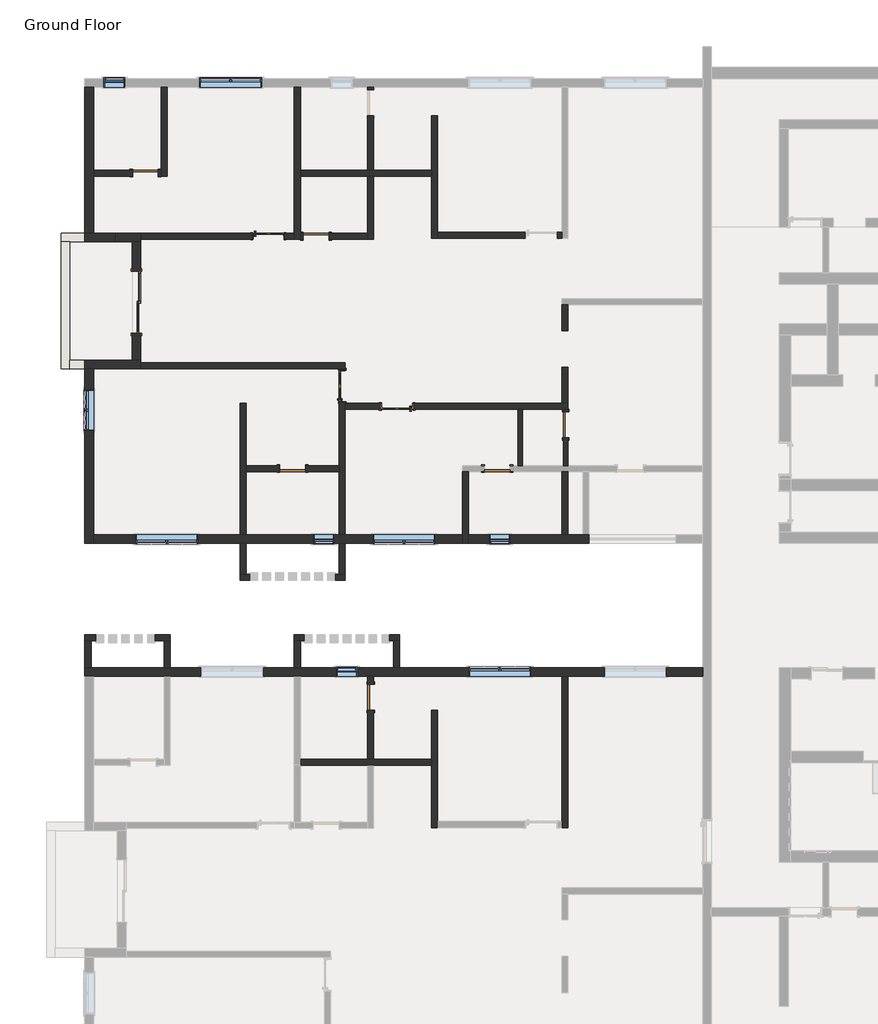
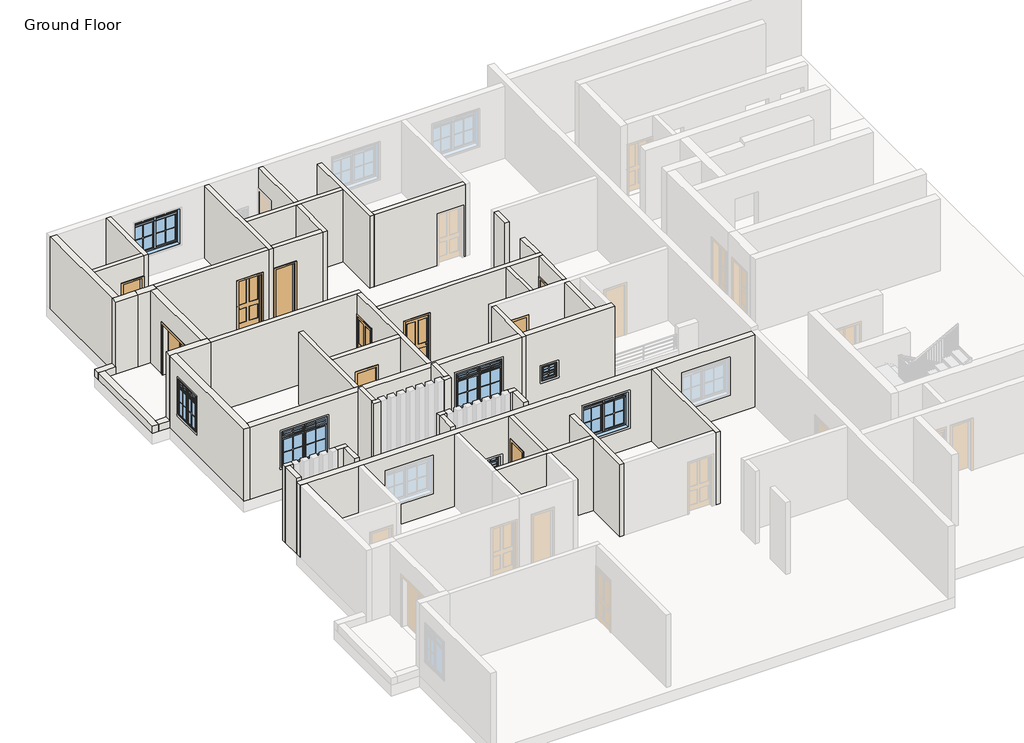
# One storey, part 2 of 9: 49 walls, 10 doors, 9 windows.
# Revit data of these elements (continued)
# Elements 13, 14, 19, 25, 28, 29, 31, 34, 38, 39, 42, 43, 46, 47 (IfcWall, "6\" INTERIOR WALL")
#   Top Offset = 0' - 0"
#   Base Offset = 0' - 0"
#   wall height = 10' - 6"
#   Phase Created = New Construction
#   Base Constraint = Ground Floor
#   Top Constraint = 1st Floor
#   Materials on its faces: "0 Cream", "Default Wall"
# Elements 15, 16, 17, 18, 20, 21, 22, 23, 24, 26, 27, 30, 32, 33, 35, 36, 37, 40, 41, 44, 45 (IfcWall, "6\" INTERIOR WALL")
#   Top Offset = 0' - 0"
#   Base Offset = 0' - 0"
#   wall height = 10' - 6"
#   Phase Created = New Construction
#   Base Constraint = Ground Floor
#   Top Constraint = 1st Floor
#   Materials on its faces: "Default Wall", "0 Cream"
# Elements 48, 49, 50, 51, 54, 55, 59 (IfcWall, "9\" EXTERIOR WALL")
#   Top Offset = 0' - 0"
#   Base Offset = 0' - 0"
#   wall height = 10' - 6"
#   Phase Created = New Construction
#   Base Constraint = Ground Floor
#   Top Constraint = 1st Floor
#   Materials on its faces: "Default Wall", "0 Cream"
# Element 52 (IfcWall, "9\" EXTERIOR WALL")
#   Top Offset = 0' - 0"
#   Base Offset = 0' - 0"
#   Unconnected Height = 1' - 0"
#   wall height = 1' - 0"
#   Phase Created = New Construction
#   Base Constraint = Ground Floor
#   Materials on its faces: "Default Wall", "0 Cream"
# Elements 53, 58 (IfcWall, "9\" EXTERIOR WALL")
#   Top Offset = 0' - 0"
#   Base Offset = 0' - 0"
#   wall height = 10' - 6"
#   Phase Created = New Construction
#   Base Constraint = Ground Floor
#   Top Constraint = 1st Floor
#   Materials on its faces: "0 Cream", "Default Wall"
# Elements 56, 57 (IfcWall, "9\" EXTERIOR WALL")
#   Top Offset = 0' - 0"
#   Base Offset = 0' - 0"
#   Unconnected Height = 1' - 0"
#   wall height = 1' - 0"
#   Phase Created = New Construction
#   Base Constraint = Ground Floor
#   Materials on its faces: "0 Cream", "Default Wall"
# Element 60 (IfcWindow, "Window-Casement-Double-Awning-Double : 4' x 5' Window")
#   Mark = "29"
#   Window Inset = 0' - 0"
#   Interior Wall Closure = 0' - 2 1/4"
#   Frame Extension = 0' - 0 1/4"
#   Exterior Wall Closure = 0' - 1 1/4"
#   Interior Trim Visibility = yes
#   Exterior Trim Visibility = yes
#   Phase Created = New Construction
#   Materials on its faces: "Wood - Stained", "Glass", "Clad - White"
# Element 61 (IfcWindow, "Window-Casement-Double-Awning-Double : 6' x 5'")
#   Mark = "5"
#   Window Inset = 0' - 0"
#   Interior Wall Closure = 0' - 2 1/4"
#   Frame Extension = 0' - 0 1/4"
#   Exterior Wall Closure = 0' - 1 1/4"
#   Interior Trim Visibility = yes
#   Exterior Trim Visibility = yes
#   Phase Created = New Construction
#   Materials on its faces: "Wood - Stained", "Glass", "Clad - White"
# Element 62 (IfcWindow, "Window-Casement-Double-Awning-Double : 6' x 5'")
#   Mark = "7"
#   Window Inset = 0' - 0"
#   Interior Wall Closure = 0' - 2 1/4"
#   Frame Extension = 0' - 0 1/4"
#   Exterior Wall Closure = 0' - 1 1/4"
#   Interior Trim Visibility = yes
#   Exterior Trim Visibility = yes
#   Phase Created = New Construction
#   Materials on its faces: "Wood - Stained", "Glass", "Clad - White"
# Element 63 (IfcWindow, "Window-Casement-Double-Awning-Double : 6' x 5'")
#   Mark = "8"
#   Window Inset = 0' - 0"
#   Interior Wall Closure = 0' - 2 1/4"
#   Frame Extension = 0' - 0 1/4"
#   Exterior Wall Closure = 0' - 1 1/4"
#   Interior Trim Visibility = yes
#   Exterior Trim Visibility = yes
#   Phase Created = New Construction
#   Materials on its faces: "Wood - Stained", "Glass", "Clad - White"
# Element 64 (IfcWindow, "Window-Casement-Double-Awning-Double : 6' x 5'")
#   Mark = "10"
#   Window Inset = 0' - 0"
#   Interior Wall Closure = 0' - 2 1/4"
#   Frame Extension = 0' - 0 1/4"
#   Exterior Wall Closure = 0' - 1 1/4"
#   Interior Trim Visibility = yes
#   Exterior Trim Visibility = yes
#   Phase Created = New Construction
#   Materials on its faces: "Wood - Stained", "Glass", "Clad - White"
# Element 65 (IfcWindow, "Window-Double-Hung")
#   Mark = "13"
#   Window Inset = 0' - 0"
#   Interior Wall Closure = 0' - 1 1/2"
#   Frame Extension = 0' - 1 1/4"
#   Exterior Wall Closure = 0' - 0 1/2"
#   Interior Trim Visibility = yes
#   Indicator Visibility = yes
#   Exterior Trim Visibility = yes
#   Phase Created = New Construction
#   Materials on its faces: "Wood - Stained", "Glass", "Clad - White"
# Element 66 (IfcWindow, "Window-Double-Hung")
#   Mark = "15"
#   Window Inset = 0' - 0"
#   Interior Wall Closure = 0' - 1 1/2"
#   Frame Extension = 0' - 1 1/4"
#   Exterior Wall Closure = 0' - 0 1/2"
#   Interior Trim Visibility = yes
#   Indicator Visibility = yes
#   Exterior Trim Visibility = yes
#   Phase Created = New Construction
#   Materials on its faces: "Wood - Stained", "Glass", "Clad - White"
# Element 67 (IfcWindow, "Window-Double-Hung")
#   Mark = "16"
#   Window Inset = 0' - 0"
#   Interior Wall Closure = 0' - 1 1/2"
#   Frame Extension = 0' - 1 1/4"
#   Exterior Wall Closure = 0' - 0 1/2"
#   Interior Trim Visibility = yes
#   Indicator Visibility = yes
#   Exterior Trim Visibility = yes
#   Phase Created = New Construction
#   Materials on its faces: "Wood - Stained", "Glass", "Clad - White"
# Element 68 (IfcWindow, "Window-Double-Hung")
#   Mark = "17"
#   Window Inset = 0' - 0"
#   Interior Wall Closure = 0' - 1 1/2"
#   Frame Extension = 0' - 1 1/4"
#   Exterior Wall Closure = 0' - 0 1/2"
#   Interior Trim Visibility = yes
#   Indicator Visibility = yes
#   Exterior Trim Visibility = yes
#   Phase Created = New Construction
#   Materials on its faces: "Wood - Stained", "Glass", "Clad - White"
# Materials
#   "Glass": class "Glass", colour RGB 0 128 192, transparency 0.75, Description = "Soda Lime Glass", Cost = 0
#   "Wood - Birch - Solid Stained Light Low Gloss": class "Wood", colour RGB 210 159 95, transparency 0, Cost = 0
#   "Paint - Sienna": colour RGB 118 70 51, transparency 0, Cost = 0
#   "Cherry": class "Wood", colour RGB 226 177 128, transparency 0, Description = "Prunus Serotina", Cost = 0
#   "Aluminum": class "Metal", colour RGB 247 247 247, transparency 0, Description = "Aluminum 6061", Cost = 0
#   "Door - Panel": class "Wood", colour RGB 210 159 95, transparency 0, Cost = 0
#   "Door - Frame": colour RGB 118 70 51, transparency 0, Cost = 0
#   "0 Cream": class "Generic", colour RGB 120 120 120, transparency 0, Cost = 0
#   "Wood - Stained": class "Wood", colour RGB 224 178 126, transparency 0, Cost = 0
#   "Clad - White": class "Wood", colour RGB 242 242 238, transparency 0, Cost = 0
#   "Default Wall": colour RGB 128 128 128, transparency 0, Cost = 0
